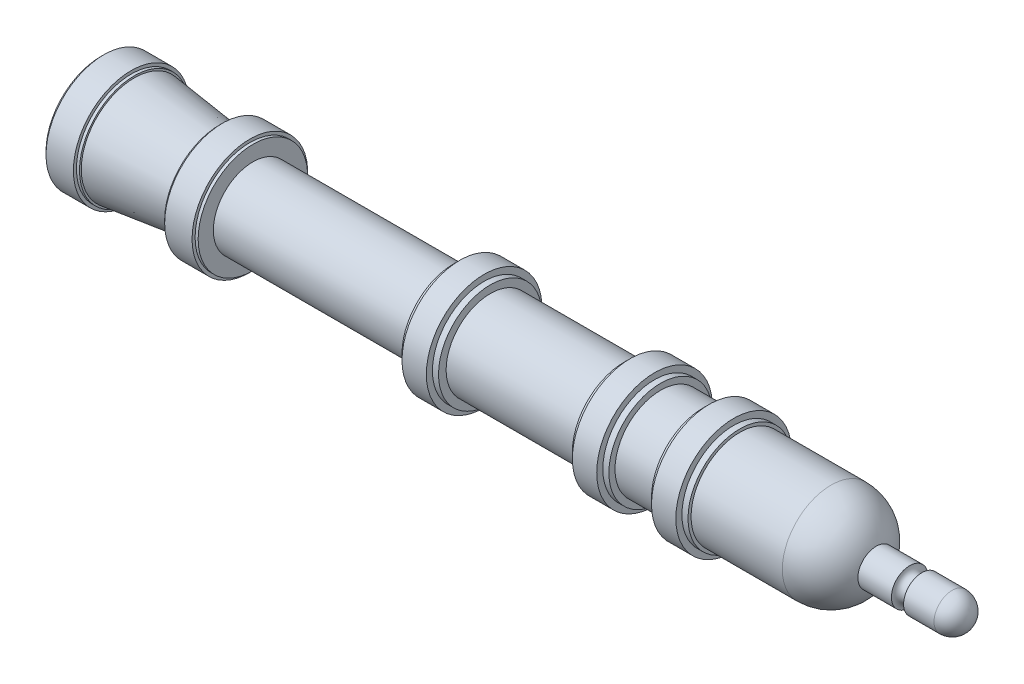
ISO-10303-21;
HEADER;
FILE_DESCRIPTION(('STEP AP214'),'2;1');
FILE_NAME('part.step','',(''),(''),'','','');
FILE_SCHEMA(('AUTOMOTIVE_DESIGN { 1 0 10303 214 1 1 1 1 }'));
ENDSEC;
DATA;
#1=APPLICATION_CONTEXT('core data for automotive mechanical design processes');
#2=APPLICATION_PROTOCOL_DEFINITION('international standard','automotive_design',2000,#1);
#3=PRODUCT_CONTEXT('',#1,'mechanical');
#4=PRODUCT('Part','Part','',(#3));
#5=PRODUCT_RELATED_PRODUCT_CATEGORY('part','',(#4));
#6=PRODUCT_DEFINITION_FORMATION('','',#4);
#7=PRODUCT_DEFINITION_CONTEXT('part definition',#1,'design');
#8=PRODUCT_DEFINITION('design','',#6,#7);
#9=PRODUCT_DEFINITION_SHAPE('','',#8);
#10=(LENGTH_UNIT() NAMED_UNIT(*) SI_UNIT(.MILLI.,.METRE.));
#11=(NAMED_UNIT(*) PLANE_ANGLE_UNIT() SI_UNIT($,.RADIAN.));
#12=(NAMED_UNIT(*) SI_UNIT($,.STERADIAN.) SOLID_ANGLE_UNIT());
#13=UNCERTAINTY_MEASURE_WITH_UNIT(LENGTH_MEASURE(1.E-05),#10,'distance_accuracy_value','');
#14=(GEOMETRIC_REPRESENTATION_CONTEXT(3) GLOBAL_UNCERTAINTY_ASSIGNED_CONTEXT((#13)) GLOBAL_UNIT_ASSIGNED_CONTEXT((#10,
#11,#12)) REPRESENTATION_CONTEXT('',''));
#15=CARTESIAN_POINT('',(0.,0.,0.));
#16=DIRECTION('',(0.,0.,1.));
#17=DIRECTION('',(1.,0.,0.));
#18=AXIS2_PLACEMENT_3D('',#15,#16,#17);
#19=CARTESIAN_POINT('',(120.,0.,0.));
#20=DIRECTION('',(-1.,0.,0.));
#21=DIRECTION('',(0.,0.,1.));
#22=AXIS2_PLACEMENT_3D('',#19,#20,#21);
#23=SPHERICAL_SURFACE('',#22,8.);
#24=CARTESIAN_POINT('',(120.,0.,0.));
#25=DIRECTION('',(-1.,0.,0.));
#26=DIRECTION('',(0.,0.,1.));
#27=AXIS2_PLACEMENT_3D('',#24,#25,#26);
#28=CIRCLE('',#27,8.);
#29=CARTESIAN_POINT('',(120.,0.,8.));
#30=VERTEX_POINT('',#29);
#31=EDGE_CURVE('E42',#30,#30,#28,.T.);
#32=ORIENTED_EDGE('',*,*,#31,.F.);
#33=EDGE_LOOP('',(#32));
#34=FACE_BOUND('',#33,.T.);
#35=CARTESIAN_POINT('',(127.416198487096,0.,0.));
#36=DIRECTION('',(-1.,0.,0.));
#37=DIRECTION('',(0.,0.,1.));
#38=AXIS2_PLACEMENT_3D('',#35,#36,#37);
#39=CIRCLE('',#38,3.);
#40=CARTESIAN_POINT('',(127.416198487096,0.,3.));
#41=VERTEX_POINT('',#40);
#42=EDGE_CURVE('E57',#41,#41,#39,.T.);
#43=ORIENTED_EDGE('',*,*,#42,.T.);
#44=EDGE_LOOP('',(#43));
#45=FACE_BOUND('',#44,.T.);
#46=ADVANCED_FACE('F40',(#34,#45),#23,.T.);
#47=CARTESIAN_POINT('',(0.,0.,0.));
#48=DIRECTION('',(1.,0.,0.));
#49=DIRECTION('',(0.,0.,-1.));
#50=AXIS2_PLACEMENT_3D('',#47,#48,#49);
#51=PLANE('',#50);
#52=CARTESIAN_POINT('',(0.,0.,0.));
#53=DIRECTION('',(-1.,0.,0.));
#54=DIRECTION('',(0.,0.,1.));
#55=AXIS2_PLACEMENT_3D('',#52,#53,#54);
#56=CIRCLE('',#55,9.);
#57=CARTESIAN_POINT('',(0.,0.,9.));
#58=VERTEX_POINT('',#57);
#59=EDGE_CURVE('E48',#58,#58,#56,.T.);
#60=ORIENTED_EDGE('',*,*,#59,.T.);
#61=EDGE_LOOP('',(#60));
#62=FACE_BOUND('',#61,.T.);
#63=ADVANCED_FACE('F267',(#62),#51,.F.);
#64=CARTESIAN_POINT('',(0.,0.,0.));
#65=DIRECTION('',(-1.,0.,0.));
#66=DIRECTION('',(0.,0.,1.));
#67=AXIS2_PLACEMENT_3D('',#64,#65,#66);
#68=CYLINDRICAL_SURFACE('',#67,9.);
#69=ORIENTED_EDGE('',*,*,#59,.F.);
#70=EDGE_LOOP('',(#69));
#71=FACE_BOUND('',#70,.T.);
#72=CARTESIAN_POINT('',(0.499999999999999,0.,0.));
#73=DIRECTION('',(-1.,0.,0.));
#74=DIRECTION('',(0.,0.,1.));
#75=AXIS2_PLACEMENT_3D('',#72,#73,#74);
#76=CIRCLE('',#75,9.);
#77=CARTESIAN_POINT('',(0.499999999999999,0.,9.));
#78=VERTEX_POINT('',#77);
#79=EDGE_CURVE('E52',#78,#78,#76,.T.);
#80=ORIENTED_EDGE('',*,*,#79,.T.);
#81=EDGE_LOOP('',(#80));
#82=FACE_BOUND('',#81,.T.);
#83=ADVANCED_FACE('F185',(#71,#82),#68,.T.);
#84=CARTESIAN_POINT('',(0.499999999999999,9.,0.));
#85=DIRECTION('',(1.,0.,0.));
#86=DIRECTION('',(0.,0.,-1.));
#87=AXIS2_PLACEMENT_3D('',#84,#85,#86);
#88=PLANE('',#87);
#89=ORIENTED_EDGE('',*,*,#79,.F.);
#90=EDGE_LOOP('',(#89));
#91=FACE_BOUND('',#90,.T.);
#92=CARTESIAN_POINT('',(0.499999999999999,0.,0.));
#93=DIRECTION('',(-1.,0.,0.));
#94=DIRECTION('',(0.,0.,1.));
#95=AXIS2_PLACEMENT_3D('',#92,#93,#94);
#96=CIRCLE('',#95,9.5);
#97=CARTESIAN_POINT('',(0.499999999999999,0.,9.5));
#98=VERTEX_POINT('',#97);
#99=EDGE_CURVE('E180',#98,#98,#96,.T.);
#100=ORIENTED_EDGE('',*,*,#99,.T.);
#101=EDGE_LOOP('',(#100));
#102=FACE_BOUND('',#101,.T.);
#103=ADVANCED_FACE('F183',(#91,#102),#88,.F.);
#104=CARTESIAN_POINT('',(0.,0.,0.));
#105=DIRECTION('',(-1.,0.,0.));
#106=DIRECTION('',(0.,0.,1.));
#107=AXIS2_PLACEMENT_3D('',#104,#105,#106);
#108=CYLINDRICAL_SURFACE('',#107,9.5);
#109=ORIENTED_EDGE('',*,*,#99,.F.);
#110=EDGE_LOOP('',(#109));
#111=FACE_BOUND('',#110,.T.);
#112=CARTESIAN_POINT('',(5.,0.,0.));
#113=DIRECTION('',(-1.,0.,0.));
#114=DIRECTION('',(0.,0.,1.));
#115=AXIS2_PLACEMENT_3D('',#112,#113,#114);
#116=CIRCLE('',#115,9.5);
#117=CARTESIAN_POINT('',(5.,0.,9.5));
#118=VERTEX_POINT('',#117);
#119=EDGE_CURVE('E172',#118,#118,#116,.T.);
#120=ORIENTED_EDGE('',*,*,#119,.T.);
#121=EDGE_LOOP('',(#120));
#122=FACE_BOUND('',#121,.T.);
#123=ADVANCED_FACE('F190',(#111,#122),#108,.T.);
#124=CARTESIAN_POINT('',(5.,9.5,0.));
#125=DIRECTION('',(-1.,0.,0.));
#126=DIRECTION('',(0.,0.,1.));
#127=AXIS2_PLACEMENT_3D('',#124,#125,#126);
#128=PLANE('',#127);
#129=ORIENTED_EDGE('',*,*,#119,.F.);
#130=EDGE_LOOP('',(#129));
#131=FACE_BOUND('',#130,.T.);
#132=CARTESIAN_POINT('',(5.,0.,0.));
#133=DIRECTION('',(-1.,0.,0.));
#134=DIRECTION('',(0.,0.,1.));
#135=AXIS2_PLACEMENT_3D('',#132,#133,#134);
#136=CIRCLE('',#135,9.);
#137=CARTESIAN_POINT('',(5.,0.,9.));
#138=VERTEX_POINT('',#137);
#139=EDGE_CURVE('E171',#138,#138,#136,.T.);
#140=ORIENTED_EDGE('',*,*,#139,.T.);
#141=EDGE_LOOP('',(#140));
#142=FACE_BOUND('',#141,.T.);
#143=ADVANCED_FACE('F194',(#131,#142),#128,.F.);
#144=CARTESIAN_POINT('',(0.,0.,0.));
#145=DIRECTION('',(-1.,0.,0.));
#146=DIRECTION('',(0.,0.,1.));
#147=AXIS2_PLACEMENT_3D('',#144,#145,#146);
#148=CYLINDRICAL_SURFACE('',#147,9.);
#149=ORIENTED_EDGE('',*,*,#139,.F.);
#150=EDGE_LOOP('',(#149));
#151=FACE_BOUND('',#150,.T.);
#152=CARTESIAN_POINT('',(5.5,0.,0.));
#153=DIRECTION('',(-1.,0.,0.));
#154=DIRECTION('',(0.,0.,1.));
#155=AXIS2_PLACEMENT_3D('',#152,#153,#154);
#156=CIRCLE('',#155,9.);
#157=CARTESIAN_POINT('',(5.5,0.,9.));
#158=VERTEX_POINT('',#157);
#159=EDGE_CURVE('E166',#158,#158,#156,.T.);
#160=ORIENTED_EDGE('',*,*,#159,.T.);
#161=EDGE_LOOP('',(#160));
#162=FACE_BOUND('',#161,.T.);
#163=ADVANCED_FACE('F196',(#151,#162),#148,.T.);
#164=CARTESIAN_POINT('',(5.5,9.,0.));
#165=DIRECTION('',(-1.,0.,0.));
#166=DIRECTION('',(0.,0.,1.));
#167=AXIS2_PLACEMENT_3D('',#164,#165,#166);
#168=PLANE('',#167);
#169=ORIENTED_EDGE('',*,*,#159,.F.);
#170=EDGE_LOOP('',(#169));
#171=FACE_BOUND('',#170,.T.);
#172=CARTESIAN_POINT('',(5.5,0.,0.));
#173=DIRECTION('',(-1.,0.,0.));
#174=DIRECTION('',(0.,0.,1.));
#175=AXIS2_PLACEMENT_3D('',#172,#173,#174);
#176=CIRCLE('',#175,8.7);
#177=CARTESIAN_POINT('',(5.5,0.,8.7));
#178=VERTEX_POINT('',#177);
#179=EDGE_CURVE('E164',#178,#178,#176,.T.);
#180=ORIENTED_EDGE('',*,*,#179,.T.);
#181=EDGE_LOOP('',(#180));
#182=FACE_BOUND('',#181,.T.);
#183=ADVANCED_FACE('F201',(#171,#182),#168,.F.);
#184=CARTESIAN_POINT('',(19.5,0.,0.));
#185=DIRECTION('',(-1.,0.,0.));
#186=DIRECTION('',(0.,0.,1.));
#187=AXIS2_PLACEMENT_3D('',#184,#185,#186);
#188=CONICAL_SURFACE('',#187,7.,0.120836979157072);
#189=ORIENTED_EDGE('',*,*,#179,.F.);
#190=EDGE_LOOP('',(#189));
#191=FACE_BOUND('',#190,.T.);
#192=CARTESIAN_POINT('',(19.5,0.,0.));
#193=DIRECTION('',(-1.,0.,0.));
#194=DIRECTION('',(0.,0.,1.));
#195=AXIS2_PLACEMENT_3D('',#192,#193,#194);
#196=CIRCLE('',#195,7.);
#197=CARTESIAN_POINT('',(19.5,0.,7.));
#198=VERTEX_POINT('',#197);
#199=EDGE_CURVE('E162',#198,#198,#196,.T.);
#200=ORIENTED_EDGE('',*,*,#199,.T.);
#201=EDGE_LOOP('',(#200));
#202=FACE_BOUND('',#201,.T.);
#203=ADVANCED_FACE('F212',(#191,#202),#188,.T.);
#204=CARTESIAN_POINT('',(19.5,7.,0.));
#205=DIRECTION('',(1.,0.,0.));
#206=DIRECTION('',(0.,0.,-1.));
#207=AXIS2_PLACEMENT_3D('',#204,#205,#206);
#208=PLANE('',#207);
#209=ORIENTED_EDGE('',*,*,#199,.F.);
#210=EDGE_LOOP('',(#209));
#211=FACE_BOUND('',#210,.T.);
#212=CARTESIAN_POINT('',(19.5,0.,0.));
#213=DIRECTION('',(-1.,0.,0.));
#214=DIRECTION('',(0.,0.,1.));
#215=AXIS2_PLACEMENT_3D('',#212,#213,#214);
#216=CIRCLE('',#215,9.);
#217=CARTESIAN_POINT('',(19.5,0.,9.));
#218=VERTEX_POINT('',#217);
#219=EDGE_CURVE('E160',#218,#218,#216,.T.);
#220=ORIENTED_EDGE('',*,*,#219,.T.);
#221=EDGE_LOOP('',(#220));
#222=FACE_BOUND('',#221,.T.);
#223=ADVANCED_FACE('F220',(#211,#222),#208,.F.);
#224=CARTESIAN_POINT('',(0.,0.,0.));
#225=DIRECTION('',(-1.,0.,0.));
#226=DIRECTION('',(0.,0.,1.));
#227=AXIS2_PLACEMENT_3D('',#224,#225,#226);
#228=CYLINDRICAL_SURFACE('',#227,9.);
#229=ORIENTED_EDGE('',*,*,#219,.F.);
#230=EDGE_LOOP('',(#229));
#231=FACE_BOUND('',#230,.T.);
#232=CARTESIAN_POINT('',(20.,0.,0.));
#233=DIRECTION('',(-1.,0.,0.));
#234=DIRECTION('',(0.,0.,1.));
#235=AXIS2_PLACEMENT_3D('',#232,#233,#234);
#236=CIRCLE('',#235,9.);
#237=CARTESIAN_POINT('',(20.,0.,9.));
#238=VERTEX_POINT('',#237);
#239=EDGE_CURVE('E158',#238,#238,#236,.T.);
#240=ORIENTED_EDGE('',*,*,#239,.T.);
#241=EDGE_LOOP('',(#240));
#242=FACE_BOUND('',#241,.T.);
#243=ADVANCED_FACE('F222',(#231,#242),#228,.T.);
#244=CARTESIAN_POINT('',(20.,9.,0.));
#245=DIRECTION('',(1.,0.,0.));
#246=DIRECTION('',(0.,0.,-1.));
#247=AXIS2_PLACEMENT_3D('',#244,#245,#246);
#248=PLANE('',#247);
#249=ORIENTED_EDGE('',*,*,#239,.F.);
#250=EDGE_LOOP('',(#249));
#251=FACE_BOUND('',#250,.T.);
#252=CARTESIAN_POINT('',(20.,0.,0.));
#253=DIRECTION('',(-1.,0.,0.));
#254=DIRECTION('',(0.,0.,1.));
#255=AXIS2_PLACEMENT_3D('',#252,#253,#254);
#256=CIRCLE('',#255,9.5);
#257=CARTESIAN_POINT('',(20.,0.,9.5));
#258=VERTEX_POINT('',#257);
#259=EDGE_CURVE('E154',#258,#258,#256,.T.);
#260=ORIENTED_EDGE('',*,*,#259,.T.);
#261=EDGE_LOOP('',(#260));
#262=FACE_BOUND('',#261,.T.);
#263=ADVANCED_FACE('F230',(#251,#262),#248,.F.);
#264=CARTESIAN_POINT('',(0.,0.,0.));
#265=DIRECTION('',(-1.,0.,0.));
#266=DIRECTION('',(0.,0.,1.));
#267=AXIS2_PLACEMENT_3D('',#264,#265,#266);
#268=CYLINDRICAL_SURFACE('',#267,9.5);
#269=ORIENTED_EDGE('',*,*,#259,.F.);
#270=EDGE_LOOP('',(#269));
#271=FACE_BOUND('',#270,.T.);
#272=CARTESIAN_POINT('',(24.5,0.,0.));
#273=DIRECTION('',(-1.,0.,0.));
#274=DIRECTION('',(0.,0.,1.));
#275=AXIS2_PLACEMENT_3D('',#272,#273,#274);
#276=CIRCLE('',#275,9.5);
#277=CARTESIAN_POINT('',(24.5,0.,9.5));
#278=VERTEX_POINT('',#277);
#279=EDGE_CURVE('E148',#278,#278,#276,.T.);
#280=ORIENTED_EDGE('',*,*,#279,.T.);
#281=EDGE_LOOP('',(#280));
#282=FACE_BOUND('',#281,.T.);
#283=ADVANCED_FACE('F232',(#271,#282),#268,.T.);
#284=CARTESIAN_POINT('',(24.5,9.5,0.));
#285=DIRECTION('',(-1.,0.,0.));
#286=DIRECTION('',(0.,0.,1.));
#287=AXIS2_PLACEMENT_3D('',#284,#285,#286);
#288=PLANE('',#287);
#289=ORIENTED_EDGE('',*,*,#279,.F.);
#290=EDGE_LOOP('',(#289));
#291=FACE_BOUND('',#290,.T.);
#292=CARTESIAN_POINT('',(24.5,0.,0.));
#293=DIRECTION('',(-1.,0.,0.));
#294=DIRECTION('',(0.,0.,1.));
#295=AXIS2_PLACEMENT_3D('',#292,#293,#294);
#296=CIRCLE('',#295,9.);
#297=CARTESIAN_POINT('',(24.5,0.,9.));
#298=VERTEX_POINT('',#297);
#299=EDGE_CURVE('E150',#298,#298,#296,.T.);
#300=ORIENTED_EDGE('',*,*,#299,.T.);
#301=EDGE_LOOP('',(#300));
#302=FACE_BOUND('',#301,.T.);
#303=ADVANCED_FACE('F241',(#291,#302),#288,.F.);
#304=CARTESIAN_POINT('',(0.,0.,0.));
#305=DIRECTION('',(-1.,0.,0.));
#306=DIRECTION('',(0.,0.,1.));
#307=AXIS2_PLACEMENT_3D('',#304,#305,#306);
#308=CYLINDRICAL_SURFACE('',#307,9.);
#309=ORIENTED_EDGE('',*,*,#299,.F.);
#310=EDGE_LOOP('',(#309));
#311=FACE_BOUND('',#310,.T.);
#312=CARTESIAN_POINT('',(25.,0.,0.));
#313=DIRECTION('',(-1.,0.,0.));
#314=DIRECTION('',(0.,0.,1.));
#315=AXIS2_PLACEMENT_3D('',#312,#313,#314);
#316=CIRCLE('',#315,9.);
#317=CARTESIAN_POINT('',(25.,0.,9.));
#318=VERTEX_POINT('',#317);
#319=EDGE_CURVE('E144',#318,#318,#316,.T.);
#320=ORIENTED_EDGE('',*,*,#319,.T.);
#321=EDGE_LOOP('',(#320));
#322=FACE_BOUND('',#321,.T.);
#323=ADVANCED_FACE('F250',(#311,#322),#308,.T.);
#324=CARTESIAN_POINT('',(25.,9.,0.));
#325=DIRECTION('',(-1.,0.,0.));
#326=DIRECTION('',(0.,0.,1.));
#327=AXIS2_PLACEMENT_3D('',#324,#325,#326);
#328=PLANE('',#327);
#329=CARTESIAN_POINT('',(25.,0.,0.));
#330=DIRECTION('',(-1.,0.,0.));
#331=DIRECTION('',(0.,0.,1.));
#332=AXIS2_PLACEMENT_3D('',#329,#330,#331);
#333=CIRCLE('',#332,6.5);
#334=CARTESIAN_POINT('',(25.,0.,6.5));
#335=VERTEX_POINT('',#334);
#336=EDGE_CURVE('E142',#335,#335,#333,.T.);
#337=ORIENTED_EDGE('',*,*,#336,.T.);
#338=EDGE_LOOP('',(#337));
#339=FACE_BOUND('',#338,.T.);
#340=ORIENTED_EDGE('',*,*,#319,.F.);
#341=EDGE_LOOP('',(#340));
#342=FACE_BOUND('',#341,.T.);
#343=ADVANCED_FACE('F254',(#339,#342),#328,.F.);
#344=CARTESIAN_POINT('',(25.,0.,0.));
#345=DIRECTION('',(-1.,0.,0.));
#346=DIRECTION('',(0.,0.,1.));
#347=AXIS2_PLACEMENT_3D('',#344,#345,#346);
#348=CYLINDRICAL_SURFACE('',#347,6.5);
#349=ORIENTED_EDGE('',*,*,#336,.F.);
#350=EDGE_LOOP('',(#349));
#351=FACE_BOUND('',#350,.T.);
#352=CARTESIAN_POINT('',(58.,0.,0.));
#353=DIRECTION('',(-1.,0.,0.));
#354=DIRECTION('',(0.,0.,1.));
#355=AXIS2_PLACEMENT_3D('',#352,#353,#354);
#356=CIRCLE('',#355,6.5);
#357=CARTESIAN_POINT('',(58.,0.,6.5));
#358=VERTEX_POINT('',#357);
#359=EDGE_CURVE('E137',#358,#358,#356,.T.);
#360=ORIENTED_EDGE('',*,*,#359,.T.);
#361=EDGE_LOOP('',(#360));
#362=FACE_BOUND('',#361,.T.);
#363=ADVANCED_FACE('F259',(#351,#362),#348,.T.);
#364=CARTESIAN_POINT('',(58.,0.,0.));
#365=DIRECTION('',(1.,0.,0.));
#366=DIRECTION('',(0.,0.,-1.));
#367=AXIS2_PLACEMENT_3D('',#364,#365,#366);
#368=PLANE('',#367);
#369=ORIENTED_EDGE('',*,*,#359,.F.);
#370=EDGE_LOOP('',(#369));
#371=FACE_BOUND('',#370,.T.);
#372=CARTESIAN_POINT('',(58.,0.,0.));
#373=DIRECTION('',(-1.,0.,0.));
#374=DIRECTION('',(0.,0.,1.));
#375=AXIS2_PLACEMENT_3D('',#372,#373,#374);
#376=CIRCLE('',#375,8.5);
#377=CARTESIAN_POINT('',(58.,0.,8.5));
#378=VERTEX_POINT('',#377);
#379=EDGE_CURVE('E133',#378,#378,#376,.T.);
#380=ORIENTED_EDGE('',*,*,#379,.T.);
#381=EDGE_LOOP('',(#380));
#382=FACE_BOUND('',#381,.T.);
#383=ADVANCED_FACE('F261',(#371,#382),#368,.F.);
#384=CARTESIAN_POINT('',(58.,0.,0.));
#385=DIRECTION('',(-1.,0.,0.));
#386=DIRECTION('',(0.,0.,1.));
#387=AXIS2_PLACEMENT_3D('',#384,#385,#386);
#388=CYLINDRICAL_SURFACE('',#387,8.5);
#389=ORIENTED_EDGE('',*,*,#379,.F.);
#390=EDGE_LOOP('',(#389));
#391=FACE_BOUND('',#390,.T.);
#392=CARTESIAN_POINT('',(59.,0.,0.));
#393=DIRECTION('',(-1.,0.,0.));
#394=DIRECTION('',(0.,0.,1.));
#395=AXIS2_PLACEMENT_3D('',#392,#393,#394);
#396=CIRCLE('',#395,8.5);
#397=CARTESIAN_POINT('',(59.,0.,8.5));
#398=VERTEX_POINT('',#397);
#399=EDGE_CURVE('E135',#398,#398,#396,.T.);
#400=ORIENTED_EDGE('',*,*,#399,.T.);
#401=EDGE_LOOP('',(#400));
#402=FACE_BOUND('',#401,.T.);
#403=ADVANCED_FACE('F362',(#391,#402),#388,.T.);
#404=CARTESIAN_POINT('',(59.,8.5,0.));
#405=DIRECTION('',(1.,0.,0.));
#406=DIRECTION('',(0.,0.,-1.));
#407=AXIS2_PLACEMENT_3D('',#404,#405,#406);
#408=PLANE('',#407);
#409=ORIENTED_EDGE('',*,*,#399,.F.);
#410=EDGE_LOOP('',(#409));
#411=FACE_BOUND('',#410,.T.);
#412=CARTESIAN_POINT('',(59.,0.,0.));
#413=DIRECTION('',(-1.,0.,0.));
#414=DIRECTION('',(0.,0.,1.));
#415=AXIS2_PLACEMENT_3D('',#412,#413,#414);
#416=CIRCLE('',#415,9.5);
#417=CARTESIAN_POINT('',(59.,0.,9.5));
#418=VERTEX_POINT('',#417);
#419=EDGE_CURVE('E126',#418,#418,#416,.T.);
#420=ORIENTED_EDGE('',*,*,#419,.T.);
#421=EDGE_LOOP('',(#420));
#422=FACE_BOUND('',#421,.T.);
#423=ADVANCED_FACE('F374',(#411,#422),#408,.F.);
#424=CARTESIAN_POINT('',(58.,0.,0.));
#425=DIRECTION('',(-1.,0.,0.));
#426=DIRECTION('',(0.,0.,1.));
#427=AXIS2_PLACEMENT_3D('',#424,#425,#426);
#428=CYLINDRICAL_SURFACE('',#427,9.5);
#429=ORIENTED_EDGE('',*,*,#419,.F.);
#430=EDGE_LOOP('',(#429));
#431=FACE_BOUND('',#430,.T.);
#432=CARTESIAN_POINT('',(63.,0.,0.));
#433=DIRECTION('',(-1.,0.,0.));
#434=DIRECTION('',(0.,0.,1.));
#435=AXIS2_PLACEMENT_3D('',#432,#433,#434);
#436=CIRCLE('',#435,9.5);
#437=CARTESIAN_POINT('',(63.,0.,9.5));
#438=VERTEX_POINT('',#437);
#439=EDGE_CURVE('E127',#438,#438,#436,.T.);
#440=ORIENTED_EDGE('',*,*,#439,.T.);
#441=EDGE_LOOP('',(#440));
#442=FACE_BOUND('',#441,.T.);
#443=ADVANCED_FACE('F383',(#431,#442),#428,.T.);
#444=CARTESIAN_POINT('',(63.,9.5,0.));
#445=DIRECTION('',(-1.,0.,0.));
#446=DIRECTION('',(0.,0.,1.));
#447=AXIS2_PLACEMENT_3D('',#444,#445,#446);
#448=PLANE('',#447);
#449=ORIENTED_EDGE('',*,*,#439,.F.);
#450=EDGE_LOOP('',(#449));
#451=FACE_BOUND('',#450,.T.);
#452=CARTESIAN_POINT('',(63.,0.,0.));
#453=DIRECTION('',(-1.,0.,0.));
#454=DIRECTION('',(0.,0.,1.));
#455=AXIS2_PLACEMENT_3D('',#452,#453,#454);
#456=CIRCLE('',#455,8.5);
#457=CARTESIAN_POINT('',(63.,0.,8.5));
#458=VERTEX_POINT('',#457);
#459=EDGE_CURVE('E124',#458,#458,#456,.T.);
#460=ORIENTED_EDGE('',*,*,#459,.T.);
#461=EDGE_LOOP('',(#460));
#462=FACE_BOUND('',#461,.T.);
#463=ADVANCED_FACE('F393',(#451,#462),#448,.F.);
#464=CARTESIAN_POINT('',(58.,0.,0.));
#465=DIRECTION('',(-1.,0.,0.));
#466=DIRECTION('',(0.,0.,1.));
#467=AXIS2_PLACEMENT_3D('',#464,#465,#466);
#468=CYLINDRICAL_SURFACE('',#467,8.5);
#469=ORIENTED_EDGE('',*,*,#459,.F.);
#470=EDGE_LOOP('',(#469));
#471=FACE_BOUND('',#470,.T.);
#472=CARTESIAN_POINT('',(64.,0.,0.));
#473=DIRECTION('',(-1.,0.,0.));
#474=DIRECTION('',(0.,0.,1.));
#475=AXIS2_PLACEMENT_3D('',#472,#473,#474);
#476=CIRCLE('',#475,8.5);
#477=CARTESIAN_POINT('',(64.,0.,8.5));
#478=VERTEX_POINT('',#477);
#479=EDGE_CURVE('E119',#478,#478,#476,.T.);
#480=ORIENTED_EDGE('',*,*,#479,.T.);
#481=EDGE_LOOP('',(#480));
#482=FACE_BOUND('',#481,.T.);
#483=ADVANCED_FACE('F403',(#471,#482),#468,.T.);
#484=CARTESIAN_POINT('',(64.,8.5,0.));
#485=DIRECTION('',(-1.,0.,0.));
#486=DIRECTION('',(0.,0.,1.));
#487=AXIS2_PLACEMENT_3D('',#484,#485,#486);
#488=PLANE('',#487);
#489=ORIENTED_EDGE('',*,*,#479,.F.);
#490=EDGE_LOOP('',(#489));
#491=FACE_BOUND('',#490,.T.);
#492=CARTESIAN_POINT('',(64.,0.,0.));
#493=DIRECTION('',(-1.,0.,0.));
#494=DIRECTION('',(0.,0.,1.));
#495=AXIS2_PLACEMENT_3D('',#492,#493,#494);
#496=CIRCLE('',#495,7.25);
#497=CARTESIAN_POINT('',(64.,0.,7.25));
#498=VERTEX_POINT('',#497);
#499=EDGE_CURVE('E120',#498,#498,#496,.T.);
#500=ORIENTED_EDGE('',*,*,#499,.T.);
#501=EDGE_LOOP('',(#500));
#502=FACE_BOUND('',#501,.T.);
#503=ADVANCED_FACE('F413',(#491,#502),#488,.F.);
#504=CARTESIAN_POINT('',(58.,0.,0.));
#505=DIRECTION('',(-1.,0.,0.));
#506=DIRECTION('',(0.,0.,1.));
#507=AXIS2_PLACEMENT_3D('',#504,#505,#506);
#508=CYLINDRICAL_SURFACE('',#507,7.25);
#509=ORIENTED_EDGE('',*,*,#499,.F.);
#510=EDGE_LOOP('',(#509));
#511=FACE_BOUND('',#510,.T.);
#512=CARTESIAN_POINT('',(86.,0.,0.));
#513=DIRECTION('',(-1.,0.,0.));
#514=DIRECTION('',(0.,0.,1.));
#515=AXIS2_PLACEMENT_3D('',#512,#513,#514);
#516=CIRCLE('',#515,7.25);
#517=CARTESIAN_POINT('',(86.,0.,7.25));
#518=VERTEX_POINT('',#517);
#519=EDGE_CURVE('E112',#518,#518,#516,.T.);
#520=ORIENTED_EDGE('',*,*,#519,.T.);
#521=EDGE_LOOP('',(#520));
#522=FACE_BOUND('',#521,.T.);
#523=ADVANCED_FACE('F424',(#511,#522),#508,.T.);
#524=CARTESIAN_POINT('',(86.,7.25,0.));
#525=DIRECTION('',(1.,0.,0.));
#526=DIRECTION('',(0.,0.,-1.));
#527=AXIS2_PLACEMENT_3D('',#524,#525,#526);
#528=PLANE('',#527);
#529=ORIENTED_EDGE('',*,*,#519,.F.);
#530=EDGE_LOOP('',(#529));
#531=FACE_BOUND('',#530,.T.);
#532=CARTESIAN_POINT('',(86.,0.,0.));
#533=DIRECTION('',(-1.,0.,0.));
#534=DIRECTION('',(0.,0.,1.));
#535=AXIS2_PLACEMENT_3D('',#532,#533,#534);
#536=CIRCLE('',#535,8.5);
#537=CARTESIAN_POINT('',(86.,0.,8.5));
#538=VERTEX_POINT('',#537);
#539=EDGE_CURVE('E111',#538,#538,#536,.T.);
#540=ORIENTED_EDGE('',*,*,#539,.T.);
#541=EDGE_LOOP('',(#540));
#542=FACE_BOUND('',#541,.T.);
#543=ADVANCED_FACE('F434',(#531,#542),#528,.F.);
#544=CARTESIAN_POINT('',(58.,0.,0.));
#545=DIRECTION('',(-1.,0.,0.));
#546=DIRECTION('',(0.,0.,1.));
#547=AXIS2_PLACEMENT_3D('',#544,#545,#546);
#548=CYLINDRICAL_SURFACE('',#547,8.5);
#549=ORIENTED_EDGE('',*,*,#539,.F.);
#550=EDGE_LOOP('',(#549));
#551=FACE_BOUND('',#550,.T.);
#552=CARTESIAN_POINT('',(87.,0.,0.));
#553=DIRECTION('',(-1.,0.,0.));
#554=DIRECTION('',(0.,0.,1.));
#555=AXIS2_PLACEMENT_3D('',#552,#553,#554);
#556=CIRCLE('',#555,8.5);
#557=CARTESIAN_POINT('',(87.,0.,8.5));
#558=VERTEX_POINT('',#557);
#559=EDGE_CURVE('E108',#558,#558,#556,.T.);
#560=ORIENTED_EDGE('',*,*,#559,.T.);
#561=EDGE_LOOP('',(#560));
#562=FACE_BOUND('',#561,.T.);
#563=ADVANCED_FACE('F444',(#551,#562),#548,.T.);
#564=CARTESIAN_POINT('',(87.,8.5,0.));
#565=DIRECTION('',(1.,0.,0.));
#566=DIRECTION('',(0.,0.,-1.));
#567=AXIS2_PLACEMENT_3D('',#564,#565,#566);
#568=PLANE('',#567);
#569=ORIENTED_EDGE('',*,*,#559,.F.);
#570=EDGE_LOOP('',(#569));
#571=FACE_BOUND('',#570,.T.);
#572=CARTESIAN_POINT('',(87.,0.,0.));
#573=DIRECTION('',(-1.,0.,0.));
#574=DIRECTION('',(0.,0.,1.));
#575=AXIS2_PLACEMENT_3D('',#572,#573,#574);
#576=CIRCLE('',#575,9.5);
#577=CARTESIAN_POINT('',(87.,0.,9.5));
#578=VERTEX_POINT('',#577);
#579=EDGE_CURVE('E102',#578,#578,#576,.T.);
#580=ORIENTED_EDGE('',*,*,#579,.T.);
#581=EDGE_LOOP('',(#580));
#582=FACE_BOUND('',#581,.T.);
#583=ADVANCED_FACE('F453',(#571,#582),#568,.F.);
#584=CARTESIAN_POINT('',(58.,0.,0.));
#585=DIRECTION('',(-1.,0.,0.));
#586=DIRECTION('',(0.,0.,1.));
#587=AXIS2_PLACEMENT_3D('',#584,#585,#586);
#588=CYLINDRICAL_SURFACE('',#587,9.5);
#589=ORIENTED_EDGE('',*,*,#579,.F.);
#590=EDGE_LOOP('',(#589));
#591=FACE_BOUND('',#590,.T.);
#592=CARTESIAN_POINT('',(91.,0.,0.));
#593=DIRECTION('',(-1.,0.,0.));
#594=DIRECTION('',(0.,0.,1.));
#595=AXIS2_PLACEMENT_3D('',#592,#593,#594);
#596=CIRCLE('',#595,9.5);
#597=CARTESIAN_POINT('',(91.,0.,9.5));
#598=VERTEX_POINT('',#597);
#599=EDGE_CURVE('E105',#598,#598,#596,.T.);
#600=ORIENTED_EDGE('',*,*,#599,.T.);
#601=EDGE_LOOP('',(#600));
#602=FACE_BOUND('',#601,.T.);
#603=ADVANCED_FACE('F461',(#591,#602),#588,.T.);
#604=CARTESIAN_POINT('',(91.,9.5,0.));
#605=DIRECTION('',(-1.,0.,0.));
#606=DIRECTION('',(0.,0.,1.));
#607=AXIS2_PLACEMENT_3D('',#604,#605,#606);
#608=PLANE('',#607);
#609=ORIENTED_EDGE('',*,*,#599,.F.);
#610=EDGE_LOOP('',(#609));
#611=FACE_BOUND('',#610,.T.);
#612=CARTESIAN_POINT('',(91.,0.,0.));
#613=DIRECTION('',(-1.,0.,0.));
#614=DIRECTION('',(0.,0.,1.));
#615=AXIS2_PLACEMENT_3D('',#612,#613,#614);
#616=CIRCLE('',#615,8.5);
#617=CARTESIAN_POINT('',(91.,0.,8.5));
#618=VERTEX_POINT('',#617);
#619=EDGE_CURVE('E100',#618,#618,#616,.T.);
#620=ORIENTED_EDGE('',*,*,#619,.T.);
#621=EDGE_LOOP('',(#620));
#622=FACE_BOUND('',#621,.T.);
#623=ADVANCED_FACE('F473',(#611,#622),#608,.F.);
#624=CARTESIAN_POINT('',(58.,0.,0.));
#625=DIRECTION('',(-1.,0.,0.));
#626=DIRECTION('',(0.,0.,1.));
#627=AXIS2_PLACEMENT_3D('',#624,#625,#626);
#628=CYLINDRICAL_SURFACE('',#627,8.5);
#629=ORIENTED_EDGE('',*,*,#619,.F.);
#630=EDGE_LOOP('',(#629));
#631=FACE_BOUND('',#630,.T.);
#632=CARTESIAN_POINT('',(92.,0.,0.));
#633=DIRECTION('',(-1.,0.,0.));
#634=DIRECTION('',(0.,0.,1.));
#635=AXIS2_PLACEMENT_3D('',#632,#633,#634);
#636=CIRCLE('',#635,8.5);
#637=CARTESIAN_POINT('',(92.,0.,8.5));
#638=VERTEX_POINT('',#637);
#639=EDGE_CURVE('E98',#638,#638,#636,.T.);
#640=ORIENTED_EDGE('',*,*,#639,.T.);
#641=EDGE_LOOP('',(#640));
#642=FACE_BOUND('',#641,.T.);
#643=ADVANCED_FACE('F481',(#631,#642),#628,.T.);
#644=CARTESIAN_POINT('',(92.,8.5,0.));
#645=DIRECTION('',(-1.,0.,0.));
#646=DIRECTION('',(0.,0.,1.));
#647=AXIS2_PLACEMENT_3D('',#644,#645,#646);
#648=PLANE('',#647);
#649=ORIENTED_EDGE('',*,*,#639,.F.);
#650=EDGE_LOOP('',(#649));
#651=FACE_BOUND('',#650,.T.);
#652=CARTESIAN_POINT('',(92.,0.,0.));
#653=DIRECTION('',(-1.,0.,0.));
#654=DIRECTION('',(0.,0.,1.));
#655=AXIS2_PLACEMENT_3D('',#652,#653,#654);
#656=CIRCLE('',#655,7.5);
#657=CARTESIAN_POINT('',(92.,0.,7.5));
#658=VERTEX_POINT('',#657);
#659=EDGE_CURVE('E92',#658,#658,#656,.T.);
#660=ORIENTED_EDGE('',*,*,#659,.T.);
#661=EDGE_LOOP('',(#660));
#662=FACE_BOUND('',#661,.T.);
#663=ADVANCED_FACE('F492',(#651,#662),#648,.F.);
#664=CARTESIAN_POINT('',(58.,0.,0.));
#665=DIRECTION('',(-1.,0.,0.));
#666=DIRECTION('',(0.,0.,1.));
#667=AXIS2_PLACEMENT_3D('',#664,#665,#666);
#668=CYLINDRICAL_SURFACE('',#667,7.5);
#669=ORIENTED_EDGE('',*,*,#659,.F.);
#670=EDGE_LOOP('',(#669));
#671=FACE_BOUND('',#670,.T.);
#672=CARTESIAN_POINT('',(99.,0.,0.));
#673=DIRECTION('',(-1.,0.,0.));
#674=DIRECTION('',(0.,0.,1.));
#675=AXIS2_PLACEMENT_3D('',#672,#673,#674);
#676=CIRCLE('',#675,7.5);
#677=CARTESIAN_POINT('',(99.,0.,7.5));
#678=VERTEX_POINT('',#677);
#679=EDGE_CURVE('E88',#678,#678,#676,.T.);
#680=ORIENTED_EDGE('',*,*,#679,.T.);
#681=EDGE_LOOP('',(#680));
#682=FACE_BOUND('',#681,.T.);
#683=ADVANCED_FACE('F504',(#671,#682),#668,.T.);
#684=CARTESIAN_POINT('',(99.,7.5,0.));
#685=DIRECTION('',(1.,0.,0.));
#686=DIRECTION('',(0.,0.,-1.));
#687=AXIS2_PLACEMENT_3D('',#684,#685,#686);
#688=PLANE('',#687);
#689=ORIENTED_EDGE('',*,*,#679,.F.);
#690=EDGE_LOOP('',(#689));
#691=FACE_BOUND('',#690,.T.);
#692=CARTESIAN_POINT('',(99.,0.,0.));
#693=DIRECTION('',(-1.,0.,0.));
#694=DIRECTION('',(0.,0.,1.));
#695=AXIS2_PLACEMENT_3D('',#692,#693,#694);
#696=CIRCLE('',#695,8.5);
#697=CARTESIAN_POINT('',(99.,0.,8.5));
#698=VERTEX_POINT('',#697);
#699=EDGE_CURVE('E90',#698,#698,#696,.T.);
#700=ORIENTED_EDGE('',*,*,#699,.T.);
#701=EDGE_LOOP('',(#700));
#702=FACE_BOUND('',#701,.T.);
#703=ADVANCED_FACE('F513',(#691,#702),#688,.F.);
#704=CARTESIAN_POINT('',(58.,0.,0.));
#705=DIRECTION('',(-1.,0.,0.));
#706=DIRECTION('',(0.,0.,1.));
#707=AXIS2_PLACEMENT_3D('',#704,#705,#706);
#708=CYLINDRICAL_SURFACE('',#707,8.5);
#709=ORIENTED_EDGE('',*,*,#699,.F.);
#710=EDGE_LOOP('',(#709));
#711=FACE_BOUND('',#710,.T.);
#712=CARTESIAN_POINT('',(100.,0.,0.));
#713=DIRECTION('',(-1.,0.,0.));
#714=DIRECTION('',(0.,0.,1.));
#715=AXIS2_PLACEMENT_3D('',#712,#713,#714);
#716=CIRCLE('',#715,8.5);
#717=CARTESIAN_POINT('',(100.,0.,8.5));
#718=VERTEX_POINT('',#717);
#719=EDGE_CURVE('E81',#718,#718,#716,.T.);
#720=ORIENTED_EDGE('',*,*,#719,.T.);
#721=EDGE_LOOP('',(#720));
#722=FACE_BOUND('',#721,.T.);
#723=ADVANCED_FACE('F523',(#711,#722),#708,.T.);
#724=CARTESIAN_POINT('',(100.,8.5,0.));
#725=DIRECTION('',(1.,0.,0.));
#726=DIRECTION('',(0.,0.,-1.));
#727=AXIS2_PLACEMENT_3D('',#724,#725,#726);
#728=PLANE('',#727);
#729=ORIENTED_EDGE('',*,*,#719,.F.);
#730=EDGE_LOOP('',(#729));
#731=FACE_BOUND('',#730,.T.);
#732=CARTESIAN_POINT('',(100.,0.,0.));
#733=DIRECTION('',(-1.,0.,0.));
#734=DIRECTION('',(0.,0.,1.));
#735=AXIS2_PLACEMENT_3D('',#732,#733,#734);
#736=CIRCLE('',#735,9.5);
#737=CARTESIAN_POINT('',(100.,0.,9.5));
#738=VERTEX_POINT('',#737);
#739=EDGE_CURVE('E82',#738,#738,#736,.T.);
#740=ORIENTED_EDGE('',*,*,#739,.T.);
#741=EDGE_LOOP('',(#740));
#742=FACE_BOUND('',#741,.T.);
#743=ADVANCED_FACE('F533',(#731,#742),#728,.F.);
#744=CARTESIAN_POINT('',(58.,0.,0.));
#745=DIRECTION('',(-1.,0.,0.));
#746=DIRECTION('',(0.,0.,1.));
#747=AXIS2_PLACEMENT_3D('',#744,#745,#746);
#748=CYLINDRICAL_SURFACE('',#747,9.5);
#749=ORIENTED_EDGE('',*,*,#739,.F.);
#750=EDGE_LOOP('',(#749));
#751=FACE_BOUND('',#750,.T.);
#752=CARTESIAN_POINT('',(104.,0.,0.));
#753=DIRECTION('',(-1.,0.,0.));
#754=DIRECTION('',(0.,0.,1.));
#755=AXIS2_PLACEMENT_3D('',#752,#753,#754);
#756=CIRCLE('',#755,9.5);
#757=CARTESIAN_POINT('',(104.,0.,9.5));
#758=VERTEX_POINT('',#757);
#759=EDGE_CURVE('E76',#758,#758,#756,.T.);
#760=ORIENTED_EDGE('',*,*,#759,.T.);
#761=EDGE_LOOP('',(#760));
#762=FACE_BOUND('',#761,.T.);
#763=ADVANCED_FACE('F543',(#751,#762),#748,.T.);
#764=CARTESIAN_POINT('',(104.,9.5,0.));
#765=DIRECTION('',(-1.,0.,0.));
#766=DIRECTION('',(0.,0.,1.));
#767=AXIS2_PLACEMENT_3D('',#764,#765,#766);
#768=PLANE('',#767);
#769=ORIENTED_EDGE('',*,*,#759,.F.);
#770=EDGE_LOOP('',(#769));
#771=FACE_BOUND('',#770,.T.);
#772=CARTESIAN_POINT('',(104.,0.,0.));
#773=DIRECTION('',(-1.,0.,0.));
#774=DIRECTION('',(0.,0.,1.));
#775=AXIS2_PLACEMENT_3D('',#772,#773,#774);
#776=CIRCLE('',#775,8.5);
#777=CARTESIAN_POINT('',(104.,0.,8.5));
#778=VERTEX_POINT('',#777);
#779=EDGE_CURVE('E71',#778,#778,#776,.T.);
#780=ORIENTED_EDGE('',*,*,#779,.T.);
#781=EDGE_LOOP('',(#780));
#782=FACE_BOUND('',#781,.T.);
#783=ADVANCED_FACE('F554',(#771,#782),#768,.F.);
#784=CARTESIAN_POINT('',(58.,0.,0.));
#785=DIRECTION('',(-1.,0.,0.));
#786=DIRECTION('',(0.,0.,1.));
#787=AXIS2_PLACEMENT_3D('',#784,#785,#786);
#788=CYLINDRICAL_SURFACE('',#787,8.5);
#789=ORIENTED_EDGE('',*,*,#779,.F.);
#790=EDGE_LOOP('',(#789));
#791=FACE_BOUND('',#790,.T.);
#792=CARTESIAN_POINT('',(105.,0.,0.));
#793=DIRECTION('',(-1.,0.,0.));
#794=DIRECTION('',(0.,0.,1.));
#795=AXIS2_PLACEMENT_3D('',#792,#793,#794);
#796=CIRCLE('',#795,8.5);
#797=CARTESIAN_POINT('',(105.,0.,8.5));
#798=VERTEX_POINT('',#797);
#799=EDGE_CURVE('E64',#798,#798,#796,.T.);
#800=ORIENTED_EDGE('',*,*,#799,.T.);
#801=EDGE_LOOP('',(#800));
#802=FACE_BOUND('',#801,.T.);
#803=ADVANCED_FACE('F564',(#791,#802),#788,.T.);
#804=CARTESIAN_POINT('',(105.,8.5,0.));
#805=DIRECTION('',(-1.,0.,0.));
#806=DIRECTION('',(0.,0.,1.));
#807=AXIS2_PLACEMENT_3D('',#804,#805,#806);
#808=PLANE('',#807);
#809=ORIENTED_EDGE('',*,*,#799,.F.);
#810=EDGE_LOOP('',(#809));
#811=FACE_BOUND('',#810,.T.);
#812=CARTESIAN_POINT('',(105.,0.,0.));
#813=DIRECTION('',(-1.,0.,0.));
#814=DIRECTION('',(0.,0.,1.));
#815=AXIS2_PLACEMENT_3D('',#812,#813,#814);
#816=CIRCLE('',#815,8.);
#817=CARTESIAN_POINT('',(105.,0.,8.));
#818=VERTEX_POINT('',#817);
#819=EDGE_CURVE('E59',#818,#818,#816,.T.);
#820=ORIENTED_EDGE('',*,*,#819,.T.);
#821=EDGE_LOOP('',(#820));
#822=FACE_BOUND('',#821,.T.);
#823=ADVANCED_FACE('F574',(#811,#822),#808,.F.);
#824=CARTESIAN_POINT('',(58.,0.,0.));
#825=DIRECTION('',(-1.,0.,0.));
#826=DIRECTION('',(0.,0.,1.));
#827=AXIS2_PLACEMENT_3D('',#824,#825,#826);
#828=CYLINDRICAL_SURFACE('',#827,8.);
#829=ORIENTED_EDGE('',*,*,#31,.T.);
#830=EDGE_LOOP('',(#829));
#831=FACE_BOUND('',#830,.T.);
#832=ORIENTED_EDGE('',*,*,#819,.F.);
#833=EDGE_LOOP('',(#832));
#834=FACE_BOUND('',#833,.T.);
#835=ADVANCED_FACE('F583',(#831,#834),#828,.T.);
#836=CARTESIAN_POINT('',(124.926812112158,0.,0.));
#837=DIRECTION('',(-1.,0.,0.));
#838=DIRECTION('',(0.,0.,1.));
#839=AXIS2_PLACEMENT_3D('',#836,#837,#838);
#840=CYLINDRICAL_SURFACE('',#839,3.);
#841=CARTESIAN_POINT('',(139.926812112158,0.,0.));
#842=DIRECTION('',(-1.,0.,0.));
#843=DIRECTION('',(0.,0.,1.));
#844=AXIS2_PLACEMENT_3D('',#841,#842,#843);
#845=CIRCLE('',#844,3.);
#846=CARTESIAN_POINT('',(139.926812112158,0.,3.));
#847=VERTEX_POINT('',#846);
#848=EDGE_CURVE('E10',#847,#847,#845,.T.);
#849=ORIENTED_EDGE('',*,*,#848,.T.);
#850=EDGE_LOOP('',(#849));
#851=FACE_BOUND('',#850,.T.);
#852=CARTESIAN_POINT('',(134.926812112158,0.,0.));
#853=DIRECTION('',(-1.,0.,0.));
#854=DIRECTION('',(0.,0.,1.));
#855=AXIS2_PLACEMENT_3D('',#852,#853,#854);
#856=CIRCLE('',#855,3.);
#857=CARTESIAN_POINT('',(134.926812112158,0.,3.));
#858=VERTEX_POINT('',#857);
#859=EDGE_CURVE('E56',#858,#858,#856,.T.);
#860=ORIENTED_EDGE('',*,*,#859,.F.);
#861=EDGE_LOOP('',(#860));
#862=FACE_BOUND('',#861,.T.);
#863=ADVANCED_FACE('F595',(#851,#862),#840,.T.);
#864=CARTESIAN_POINT('',(133.926812112158,0.,0.));
#865=DIRECTION('',(-1.,0.,0.));
#866=DIRECTION('',(0.,0.,1.));
#867=AXIS2_PLACEMENT_3D('',#864,#865,#866);
#868=TOROIDAL_SURFACE('',#867,3.,1.);
#869=CARTESIAN_POINT('',(132.926812112158,0.,0.));
#870=DIRECTION('',(-1.,0.,0.));
#871=DIRECTION('',(0.,0.,1.));
#872=AXIS2_PLACEMENT_3D('',#869,#870,#871);
#873=CIRCLE('',#872,3.);
#874=CARTESIAN_POINT('',(132.926812112158,0.,3.));
#875=VERTEX_POINT('',#874);
#876=EDGE_CURVE('E67',#875,#875,#873,.T.);
#877=ORIENTED_EDGE('',*,*,#876,.F.);
#878=EDGE_LOOP('',(#877));
#879=FACE_BOUND('',#878,.T.);
#880=ORIENTED_EDGE('',*,*,#859,.T.);
#881=EDGE_LOOP('',(#880));
#882=FACE_BOUND('',#881,.T.);
#883=ADVANCED_FACE('F608',(#879,#882),#868,.F.);
#884=CARTESIAN_POINT('',(124.926812112158,0.,0.));
#885=DIRECTION('',(-1.,0.,0.));
#886=DIRECTION('',(0.,0.,1.));
#887=AXIS2_PLACEMENT_3D('',#884,#885,#886);
#888=CYLINDRICAL_SURFACE('',#887,3.);
#889=ORIENTED_EDGE('',*,*,#42,.F.);
#890=EDGE_LOOP('',(#889));
#891=FACE_BOUND('',#890,.T.);
#892=ORIENTED_EDGE('',*,*,#876,.T.);
#893=EDGE_LOOP('',(#892));
#894=FACE_BOUND('',#893,.T.);
#895=ADVANCED_FACE('F621',(#891,#894),#888,.T.);
#896=CARTESIAN_POINT('',(139.926812112158,0.,0.));
#897=DIRECTION('',(-1.,0.,0.));
#898=DIRECTION('',(0.,0.,1.));
#899=AXIS2_PLACEMENT_3D('',#896,#897,#898);
#900=SPHERICAL_SURFACE('',#899,3.);
#901=ORIENTED_EDGE('',*,*,#848,.F.);
#902=EDGE_LOOP('',(#901));
#903=FACE_BOUND('',#902,.T.);
#904=ADVANCED_FACE('F39',(#903),#900,.T.);
#905=CLOSED_SHELL('',(#46,#63,#83,#103,#123,#143,#163,#183,#203,#223,#243,#263,#283,#303,#323,
#343,#363,#383,#403,#423,#443,#463,#483,#503,#523,#543,#563,#583,#603,#623,#643,#663,#683,#703,
#723,#743,#763,#783,#803,#823,#835,#863,#883,#895,#904));
#906=MANIFOLD_SOLID_BREP('B2',#905);
#907=ADVANCED_BREP_SHAPE_REPRESENTATION('',(#18,#906),#14);
#908=SHAPE_DEFINITION_REPRESENTATION(#9,#907);
ENDSEC;
END-ISO-10303-21;
